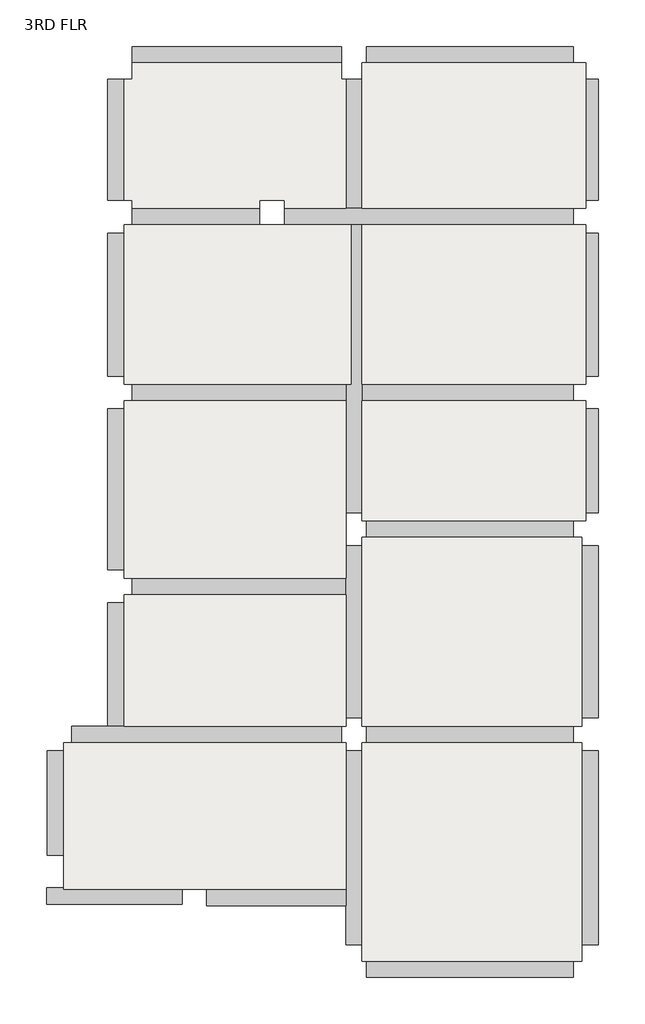
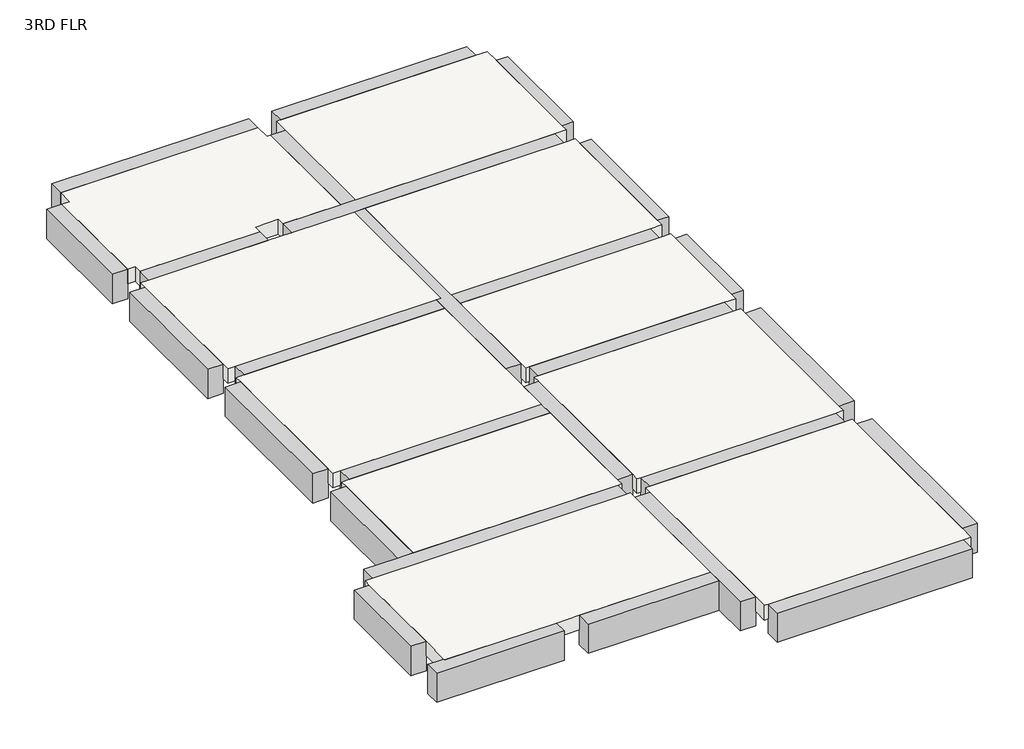
# One storey: 27 beams, 10 slabs.
"""IFC4 building model written with IfcOpenShell, lengths in millimetres."""

from ifc_helpers import new_model, si_unit, frame, origin, place, context, project, spatial, polyline, outline, extrude, faceted_brep, element, save

model = new_model("IFC4")

# Units and contexts
model_context = context("Model", 3, world=origin())
ifc_project = project(units=[si_unit("LENGTHUNIT", "METRE", prefix="MILLI")], contexts=[model_context])

# Site, building, storey
site = spatial("IfcSite", under=ifc_project)
building = spatial("IfcBuilding", under=site)
storey = spatial("IfcBuildingStorey", under=building, Name="3RD FLR", Elevation=9096.0)

# Beams
placement = place(None, origin())
element("IfcBeam", 1, ObjectType="M_Concrete-Rectangular Beam : 300 x 600mm", at=placement, inside=storey, context=model_context, shape_type="Brep", body=[
    faceted_brep([(-2096.635935, 10150.0657956, 9096.0), (-2096.635935, 10450.0657956, 9096.0), (-5925.9642664, 10450.0657956, 9096.0), (-5925.9642664, 10150.0657956, 9096.0), (-2096.635935, 10150.0657956, 8496.0), (-2096.635935, 10150.0657956, 8796.0), (-5925.9642664, 10150.0657956, 8796.0), (-5925.9642664, 10150.0657956, 8496.0), (-2096.635935, 10450.0657956, 8496.0), (-5925.9642664, 10450.0657956, 8496.0)], [[[0, 1, 2, 3]], [[4, 5, 0, 3, 6, 7]], [[8, 4, 7, 9]], [[1, 8, 9, 2]], [[2, 9, 7, 6, 3]], [[1, 0, 5, 4, 8]]]),
])
element("IfcBeam", 2, ObjectType="M_Concrete-Rectangular Beam : 300 x 600mm", at=placement, inside=storey, context=model_context, shape_type="SweptSolid", body=[
    extrude(outline(polyline([(2143.5134108, 10450.0657956), (2143.5134108, 10150.0657956), (-1646.635935, 10150.0657956), (-1646.635935, 10450.0657956), (2143.5134108, 10450.0657956)])), frame((0.0, 0.0, 8496.0), z_axis=(0.0, 0.0, 1.0), x_axis=(1.0, 0.0, 0.0)), (0.0, 0.0, 1.0), 600.0),
])
element("IfcBeam", 3, ObjectType="M_Concrete-Rectangular Beam : 300 x 600mm", at=placement, inside=storey, context=model_context, shape_type="Brep", body=[
    faceted_brep([(-6375.9642664, 7641.506653, 9096.0), (-6075.9642664, 7641.506653, 9096.0), (-6075.9642664, 9850.0657956, 9096.0), (-6375.9642664, 9850.0657956, 9096.0), (-6375.9642664, 7641.506653, 8496.0), (-6375.9642664, 9850.0657956, 8496.0), (-6075.9642664, 7641.506653, 8496.0), (-6075.9642664, 9850.0657956, 8496.0), (-6075.9642664, 7641.506653, 8796.0), (-6075.9642664, 9850.0657956, 8796.0)], [[[0, 1, 2, 3]], [[4, 0, 3, 5]], [[6, 4, 5, 7]], [[1, 8, 6, 7, 9, 2]], [[2, 9, 7, 5, 3]], [[1, 0, 4, 6, 8]]]),
])
element("IfcBeam", 4, ObjectType="M_Concrete-Rectangular Beam : 300 x 600mm", at=placement, inside=storey, context=model_context, shape_type="SweptSolid", body=[
    extrude(outline(polyline([(-6075.9642664, 4424.5351605), (-6375.9642664, 4424.5351605), (-6375.9642664, 7041.506653), (-6075.9642664, 7041.506653), (-6075.9642664, 4424.5351605)])), frame((0.0, 0.0, 8496.0), z_axis=(0.0, 0.0, 1.0), x_axis=(1.0, 0.0, 0.0)), (0.0, 0.0, 1.0), 600.0),
])
element("IfcBeam", 5, ObjectType="M_Concrete-Rectangular Beam : 300 x 600mm", at=placement, inside=storey, context=model_context, shape_type="SweptSolid", body=[
    extrude(outline(polyline([(-6075.9642664, 881.5941646), (-6375.9642664, 881.5941646), (-6375.9642664, 3824.5351605), (-6075.9642664, 3824.5351605), (-6075.9642664, 881.5941646)])), frame((0.0, 0.0, 8496.0), z_axis=(0.0, 0.0, 1.0), x_axis=(1.0, 0.0, 0.0)), (0.0, 0.0, 1.0), 600.0),
])
element("IfcBeam", 6, ObjectType="M_Concrete-Rectangular Beam : 300 x 600mm", at=placement, inside=storey, context=model_context, shape_type="SweptSolid", body=[
    extrude(outline(polyline([(2143.5134108, -6267.3380763), (2143.5134108, -6567.3380763), (-1646.635935, -6567.3380763), (-1646.635935, -6267.3380763), (2143.5134108, -6267.3380763)])), frame((0.0, 0.0, 8496.0), z_axis=(0.0, 0.0, 1.0), x_axis=(1.0, 0.0, 0.0)), (0.0, 0.0, 1.0), 600.0),
])
element("IfcBeam", 7, ObjectType="M_Concrete-Rectangular Beam : 300 x 600mm", at=placement, inside=storey, context=model_context, shape_type="SweptSolid", body=[
    extrude(outline(polyline([(2293.5134108, -2423.3693625), (2593.5134108, -2423.3693625), (2593.5134108, -5967.3380763), (2293.5134108, -5967.3380763), (2293.5134108, -2423.3693625)])), frame((0.0, 0.0, 8496.0), z_axis=(0.0, 0.0, 1.0), x_axis=(1.0, 0.0, 0.0)), (0.0, 0.0, 1.0), 600.0),
])
element("IfcBeam", 8, ObjectType="M_Concrete-Rectangular Beam : 300 x 600mm", at=placement, inside=storey, context=model_context, shape_type="SweptSolid", body=[
    extrude(outline(polyline([(2293.5134108, 1328.1057379), (2593.5134108, 1328.1057379), (2593.5134108, -1823.3693625), (2293.5134108, -1823.3693625), (2293.5134108, 1328.1057379)])), frame((0.0, 0.0, 8496.0), z_axis=(0.0, 0.0, 1.0), x_axis=(1.0, 0.0, 0.0)), (0.0, 0.0, 1.0), 600.0),
])
element("IfcBeam", 9, ObjectType="M_Concrete-Rectangular Beam : 300 x 600mm", at=placement, inside=storey, context=model_context, shape_type="SweptSolid", body=[
    extrude(outline(polyline([(8496.0, 2293.5134108), (8496.0, 2593.5134108), (9096.0, 2593.5134108), (9096.0, 2368.5134108), (8796.0, 2368.5134108), (8796.0, 2293.5134108), (8496.0, 2293.5134108)])), frame((0.0, 1928.1057379, 0.0), z_axis=(0.0, 1.0, 0.0), x_axis=(0.0, 0.0, 1.0)), (0.0, 0.0, 1.0), 1896.4294226),
])
element("IfcBeam", 10, ObjectType="M_Concrete-Rectangular Beam : 300 x 600mm", at=placement, inside=storey, context=model_context, shape_type="SweptSolid", body=[
    extrude(outline(polyline([(8496.0, 2293.5134108), (8496.0, 2593.5134108), (9096.0, 2593.5134108), (9096.0, 2368.5134108), (8796.0, 2368.5134108), (8796.0, 2293.5134108), (8496.0, 2293.5134108)])), frame((0.0, 4424.5351605, 0.0), z_axis=(0.0, 1.0, 0.0), x_axis=(0.0, 0.0, 1.0)), (0.0, 0.0, 1.0), 2616.9714925),
])
element("IfcBeam", 11, ObjectType="M_Concrete-Rectangular Beam : 300 x 600mm", at=placement, inside=storey, context=model_context, shape_type="SweptSolid", body=[
    extrude(outline(polyline([(8496.0, 2293.5134108), (8496.0, 2593.5134108), (9096.0, 2593.5134108), (9096.0, 2368.5134108), (8796.0, 2368.5134108), (8796.0, 2293.5134108), (8496.0, 2293.5134108)])), frame((0.0, 7641.506653, 0.0), z_axis=(0.0, 1.0, 0.0), x_axis=(0.0, 0.0, 1.0)), (0.0, 0.0, 1.0), 2208.5591426),
])
element("IfcBeam", 12, ObjectType="M_Concrete-Rectangular Beam : 300 x 600mm", at=placement, inside=storey, context=model_context, shape_type="Brep", body=[
    faceted_brep([(-3596.635935, 7191.506653, 9096.0), (-3596.635935, 7491.506653, 9096.0), (-5925.9642664, 7491.506653, 9096.0), (-5925.9642664, 7191.506653, 9096.0), (-3596.635935, 7191.506653, 8496.0), (-5925.9642664, 7191.506653, 8496.0), (-3596.635935, 7491.506653, 8496.0), (-5925.9642664, 7491.506653, 8496.0), (-3596.635935, 7491.506653, 8796.0), (-5925.9642664, 7491.506653, 8796.0)], [[[0, 1, 2, 3]], [[4, 0, 3, 5]], [[6, 4, 5, 7]], [[1, 8, 6, 7, 9, 2]], [[2, 9, 7, 5, 3]], [[1, 0, 4, 6, 8]]]),
])
element("IfcBeam", 13, ObjectType="M_Concrete-Rectangular Beam : 300 x 600mm", at=placement, inside=storey, context=model_context, shape_type="Brep", body=[
    faceted_brep([(-3146.635935, 7491.506653, 9096.0), (-3146.635935, 7191.506653, 9096.0), (-1928.7254278, 7191.506653, 9096.0), (-1721.635935, 7191.506653, 9096.0), (2143.5134108, 7191.506653, 9096.0), (2143.5134108, 7491.506653, 9096.0), (-1721.635935, 7491.506653, 9096.0), (-2021.635935, 7491.506653, 9096.0), (-3146.635935, 7491.506653, 8496.0), (-3146.635935, 7491.506653, 8796.0), (2143.5134108, 7491.506653, 8496.0), (-1721.635935, 7491.506653, 8496.0), (-2021.635935, 7491.506653, 8496.0), (-3146.635935, 7191.506653, 8496.0), (2143.5134108, 7191.506653, 8496.0), (-1721.635935, 7191.506653, 8496.0), (-2021.635935, 7191.506653, 8496.0)], [[[0, 1, 2, 3, 4, 5, 6, 7]], [[8, 9, 0, 7, 6, 5, 10, 11, 12]], [[13, 8, 12, 11, 10, 14, 15, 16]], [[1, 13, 16, 15, 14, 4, 3, 2]], [[1, 0, 9, 8, 13]], [[4, 14, 10, 5]]]),
])
element("IfcBeam", 14, ObjectType="M_Concrete-Rectangular Beam : 300 x 600mm", at=placement, inside=storey, context=model_context, shape_type="SweptSolid", body=[
    extrude(outline(polyline([(-1646.635935, 1478.1057379), (-1646.635935, 1778.1057379), (2143.5134108, 1778.1057379), (2143.5134108, 1478.1057379), (-1646.635935, 1478.1057379)])), frame((0.0, 0.0, 8496.0), z_axis=(0.0, 0.0, 1.0), x_axis=(1.0, 0.0, 0.0)), (0.0, 0.0, 1.0), 600.0),
])
element("IfcBeam", 15, ObjectType="M_Concrete-Rectangular Beam : 300 x 600mm", at=placement, inside=storey, context=model_context, shape_type="SweptSolid", body=[
    extrude(outline(polyline([(-1646.635935, -2273.3693625), (-1646.635935, -1973.3693625), (2143.5134108, -1973.3693625), (2143.5134108, -2273.3693625), (-1646.635935, -2273.3693625)])), frame((0.0, 0.0, 8496.0), z_axis=(0.0, 0.0, 1.0), x_axis=(1.0, 0.0, 0.0)), (0.0, 0.0, 1.0), 600.0),
])
element("IfcBeam", 16, ObjectType="M_Concrete-Rectangular Beam : 300 x 600mm", at=placement, inside=storey, context=model_context, shape_type="Brep", body=[
    faceted_brep([(-1721.635935, -2423.3693625, 9096.0), (-2021.635935, -2423.3693625, 9096.0), (-2021.635935, -4959.2575036, 9096.0), (-2021.635935, -5259.2575036, 9096.0), (-2021.635935, -5967.3380763, 9096.0), (-1721.635935, -5967.3380763, 9096.0), (-1721.635935, -2423.3693625, 8496.0), (-1721.635935, -5967.3380763, 8496.0), (-2021.635935, -2423.3693625, 8496.0), (-2021.635935, -5967.3380763, 8496.0), (-2021.635935, -5259.2575036, 8496.0), (-2021.635935, -4959.2575036, 8496.0)], [[[0, 1, 2, 3, 4, 5]], [[6, 0, 5, 7]], [[8, 6, 7, 9, 10, 11]], [[1, 8, 11, 10, 9, 4, 3, 2]], [[1, 0, 6, 8]], [[4, 9, 7, 5]]]),
])
element("IfcBeam", 17, ObjectType="M_Concrete-Rectangular Beam : 300 x 600mm", at=placement, inside=storey, context=model_context, shape_type="Brep", body=[
    faceted_brep([(-1721.635935, 1328.1057379, 9096.0), (-2021.635935, 1328.1057379, 9096.0), (-2021.635935, 731.5941646, 9096.0), (-2021.635935, 431.5941646, 9096.0), (-2021.635935, -1823.3693625, 9096.0), (-1721.635935, -1823.3693625, 9096.0), (-1721.635935, 1328.1057379, 8496.0), (-1721.635935, -1823.3693625, 8496.0), (-2021.635935, 1328.1057379, 8496.0), (-2021.635935, -1823.3693625, 8496.0), (-2021.635935, 431.5941646, 8496.0), (-2021.635935, 731.5941646, 8496.0)], [[[0, 1, 2, 3, 4, 5]], [[6, 0, 5, 7]], [[8, 6, 7, 9, 10, 11]], [[1, 8, 11, 10, 9, 4, 3, 2]], [[1, 0, 6, 8]], [[4, 9, 7, 5]]]),
])
element("IfcBeam", 18, ObjectType="M_Concrete-Rectangular Beam : 300 x 600mm", at=placement, inside=storey, context=model_context, shape_type="Brep", body=[
    faceted_brep([(-4566.635935, -4959.2575036, 9096.0), (-4566.635935, -5259.2575036, 9096.0), (-2021.635935, -5259.2575036, 9096.0), (-2021.635935, -4959.2575036, 9096.0), (-4566.635935, -5259.2575036, 8496.0), (-2021.635935, -5259.2575036, 8496.0), (-4566.635935, -4959.2575036, 8496.0), (-2021.635935, -4959.2575036, 8496.0), (-2021.635935, -4959.2575036, 8796.0)], [[[0, 1, 2, 3]], [[1, 4, 5, 2]], [[4, 6, 7, 5]], [[6, 0, 3, 8, 7]], [[0, 6, 4, 1]], [[3, 2, 5, 7, 8]]]),
])
element("IfcBeam", 19, ObjectType="M_Concrete-Rectangular Beam : 300 x 600mm", at=placement, inside=storey, context=model_context, shape_type="Brep", body=[
    faceted_brep([(-7032.9642664, -1973.3693625, 9096.0), (-7032.9642664, -2273.3693625, 9096.0), (-2096.635935, -2273.3693625, 9096.0), (-2096.635935, -1973.3693625, 9096.0), (-6075.9642664, -1973.3693625, 9096.0), (-6375.9642664, -1973.3693625, 9096.0), (-7032.9642664, -1973.3693625, 8496.0), (-2096.635935, -1973.3693625, 8496.0), (-6075.9642664, -1973.3693625, 8496.0), (-6375.9642664, -1973.3693625, 8496.0), (-7032.9642664, -2273.3693625, 8496.0), (-2096.635935, -2273.3693625, 8496.0)], [[[0, 1, 2, 3, 4, 5]], [[6, 0, 5, 4, 3, 7, 8, 9]], [[10, 6, 9, 8, 7, 11]], [[1, 10, 11, 2]], [[2, 11, 7, 3]], [[1, 0, 6, 10]]]),
])
element("IfcBeam", 20, ObjectType="M_Concrete-Rectangular Beam : 300 x 600mm", at=placement, inside=storey, context=model_context, shape_type="Brep", body=[
    faceted_brep([(-6075.9642664, 281.5941646, 9096.0), (-6375.9642664, 281.5941646, 9096.0), (-6375.9642664, -1973.3693625, 9096.0), (-6075.9642664, -1973.3693625, 9096.0), (-6375.9642664, 281.5941646, 8496.0), (-6375.9642664, -1973.3693625, 8496.0), (-6075.9642664, 281.5941646, 8496.0), (-6075.9642664, -1973.3693625, 8496.0), (-6075.9642664, -1973.3693625, 8796.0)], [[[0, 1, 2, 3]], [[1, 4, 5, 2]], [[4, 6, 7, 5]], [[6, 0, 3, 8, 7]], [[0, 6, 4, 1]], [[3, 2, 5, 7, 8]]]),
])
element("IfcBeam", 21, ObjectType="M_Concrete-Rectangular Beam : 300 x 600mm", at=placement, inside=storey, context=model_context, shape_type="SweptSolid", body=[
    extrude(outline(polyline([(-7182.9642664, -4329.2575036), (-7482.9642664, -4329.2575036), (-7482.9642664, -2423.3693625), (-7182.9642664, -2423.3693625), (-7182.9642664, -4329.2575036)])), frame((0.0, 0.0, 8496.0), z_axis=(0.0, 0.0, 1.0), x_axis=(1.0, 0.0, 0.0)), (0.0, 0.0, 1.0), 600.0),
])
element("IfcBeam", 22, ObjectType="M_Concrete-Rectangular Beam : 300 x 600mm", at=placement, inside=storey, context=model_context, shape_type="Brep", body=[
    faceted_brep([(-7496.635935, -5229.2575036, 9096.0), (-7496.635935, -4929.2575036, 9096.0), (-7496.635935, -4929.2575036, 8496.0), (-7496.635935, -5229.2575036, 8496.0), (-5016.635935, -5229.2575036, 9096.0), (-5016.635935, -4959.2575036, 9096.0), (-7182.9642664, -4959.2575036, 9096.0), (-7182.9642664, -4929.2575036, 9096.0), (-7482.9642664, -4929.2575036, 9096.0), (-7182.9642664, -4929.2575036, 8796.0), (-7032.9642664, -4929.2575036, 8796.0), (-5016.635935, -4929.2575036, 8796.0), (-5016.635935, -4929.2575036, 8496.0), (-5016.635935, -5229.2575036, 8496.0), (-5016.635935, -4959.2575036, 8796.0), (-7182.9642664, -4959.2575036, 8796.0)], [[[0, 1, 2, 3]], [[1, 0, 4, 5, 6, 7, 8]], [[2, 1, 8, 7, 9, 10, 11, 12]], [[3, 2, 12, 13]], [[0, 3, 13, 4]], [[4, 13, 12, 11, 14, 5]], [[9, 15, 14, 11, 10]], [[15, 6, 5, 14]], [[6, 15, 9, 7]]]),
])
element("IfcBeam", 23, ObjectType="M_Concrete-Rectangular Beam : 300 x 600mm", at=placement, inside=storey, context=model_context, shape_type="Brep", body=[
    faceted_brep([(-1721.635935, 9850.0657956, 9096.0), (-2021.635935, 9850.0657956, 9096.0), (-2021.635935, 7491.506653, 9096.0), (-1721.635935, 7491.506653, 9096.0), (-2021.635935, 9850.0657956, 8796.0), (-2021.635935, 9850.0657956, 8496.0), (-2021.635935, 7491.506653, 8496.0), (-2021.635935, 7491.506653, 8796.0), (-1721.635935, 9850.0657956, 8496.0), (-1721.635935, 7491.506653, 8496.0), (-1721.635935, 7491.506653, 8796.0)], [[[0, 1, 2, 3]], [[1, 4, 5, 6, 7, 2]], [[5, 8, 9, 6]], [[8, 0, 3, 10, 9]], [[0, 8, 5, 4, 1]], [[3, 2, 7, 6, 9, 10]]]),
])
element("IfcBeam", 24, ObjectType="M_Concrete-Rectangular Beam : 300 x 600mm", at=placement, inside=storey, context=model_context, shape_type="Brep", body=[
    faceted_brep([(-2021.635935, 1928.1057379, 9096.0), (-1721.635935, 1928.1057379, 9096.0), (-1721.635935, 3974.5351605, 9096.0), (-1721.635935, 4274.5351605, 9096.0), (-1721.635935, 7191.506653, 9096.0), (-1928.7254278, 7191.506653, 9096.0), (-1928.7254278, 4274.5351605, 9096.0), (-2021.635935, 4274.5351605, 9096.0), (-2021.635935, 3974.5351605, 9096.0), (-1721.635935, 1928.1057379, 8496.0), (-1721.635935, 3974.5351605, 8496.0), (-1721.635935, 4274.5351605, 8496.0), (-1721.635935, 7191.506653, 8496.0), (-1721.635935, 7191.506653, 8796.0), (-2021.635935, 1928.1057379, 8496.0), (-2021.635935, 3974.5351605, 8496.0), (-2021.635935, 4274.5351605, 8496.0), (-2021.635935, 7191.506653, 8496.0), (-2021.635935, 4274.5351605, 8796.0), (-2021.635935, 7191.506653, 8796.0), (-1928.7254278, 7191.506653, 8796.0), (-1928.7254278, 4274.5351605, 8796.0)], [[[0, 1, 2, 3, 4, 5, 6, 7, 8]], [[1, 9, 10, 11, 12, 13, 4, 3, 2]], [[9, 14, 15, 16, 17, 12, 11, 10]], [[14, 0, 8, 7, 18, 19, 17, 16, 15]], [[0, 14, 9, 1]], [[4, 13, 12, 17, 19, 20, 5]], [[21, 20, 19, 18]], [[20, 21, 6, 5]], [[6, 21, 18, 7]]]),
])
element("IfcBeam", 25, ObjectType="M_Concrete-Rectangular Beam : 300 x 600mm", at=placement, inside=storey, context=model_context, shape_type="Brep", body=[
    faceted_brep([(-5925.9642664, 731.5941646, 9096.0), (-5925.9642664, 431.5941646, 9096.0), (-2021.635935, 431.5941646, 9096.0), (-2021.635935, 731.5941646, 9096.0), (-5925.9642664, 431.5941646, 8496.0), (-2021.635935, 431.5941646, 8496.0), (-2021.635935, 431.5941646, 8796.0), (-5925.9642664, 731.5941646, 8496.0), (-2021.635935, 731.5941646, 8496.0), (-2021.635935, 731.5941646, 8796.0)], [[[0, 1, 2, 3]], [[1, 4, 5, 6, 2]], [[4, 7, 8, 5]], [[7, 0, 3, 9, 8]], [[0, 7, 4, 1]], [[3, 2, 6, 5, 8, 9]]]),
])
element("IfcBeam", 26, ObjectType="M_Concrete-Rectangular Beam : 300 x 600mm", at=placement, inside=storey, context=model_context, shape_type="Brep", body=[
    faceted_brep([(-5925.9642664, 4274.5351605, 9096.0), (-5925.9642664, 3974.5351605, 9096.0), (-2021.635935, 3974.5351605, 9096.0), (-2021.635935, 4274.5351605, 9096.0), (-5925.9642664, 3974.5351605, 8496.0), (-2021.635935, 3974.5351605, 8496.0), (-2021.635935, 3974.5351605, 8796.0), (-5925.9642664, 4274.5351605, 8496.0), (-2021.635935, 4274.5351605, 8496.0), (-2021.635935, 4274.5351605, 8796.0)], [[[0, 1, 2, 3]], [[1, 4, 5, 6, 2]], [[4, 7, 8, 5]], [[7, 0, 3, 9, 8]], [[0, 7, 4, 1]], [[3, 2, 6, 5, 8, 9]]]),
])
element("IfcBeam", 27, ObjectType="M_Concrete-Rectangular Beam : 300 x 600mm", at=placement, inside=storey, context=model_context, shape_type="Brep", body=[
    faceted_brep([(2143.5134108, 3974.5351605, 9096.0), (2143.5134108, 4274.5351605, 9096.0), (-1721.635935, 4274.5351605, 9096.0), (-1721.635935, 3974.5351605, 9096.0), (2143.5134108, 4274.5351605, 8496.0), (-1721.635935, 4274.5351605, 8496.0), (-1721.635935, 4274.5351605, 8796.0), (2143.5134108, 3974.5351605, 8496.0), (-1721.635935, 3974.5351605, 8496.0), (-1721.635935, 3974.5351605, 8796.0)], [[[0, 1, 2, 3]], [[1, 4, 5, 6, 2]], [[4, 7, 8, 5]], [[7, 0, 3, 9, 8]], [[0, 7, 4, 1]], [[3, 2, 6, 5, 8, 9]]]),
])

# Slabs
element("IfcSlab", 28, ObjectType="Generic 300mm", at=placement, inside=storey, context=model_context, shape_type="SweptSolid", body=[
    extrude(outline(polyline([(-2096.635935, 10150.0657956), (-2096.635935, 9850.0657956), (-2021.635935, 9850.0657956), (-2021.635935, 7491.506653), (-3146.635935, 7491.506653), (-3146.635935, 7641.506653), (-3596.635935, 7641.506653), (-3596.635935, 7491.506653), (-5925.9642664, 7491.506653), (-5925.9642664, 7641.506653), (-6075.9642664, 7641.506653), (-6075.9642664, 9850.0657956), (-5925.9642664, 9850.0657956), (-5925.9642664, 10150.0657956), (-2096.635935, 10150.0657956)])), frame((0.0, 0.0, 8796.0), z_axis=(0.0, 0.0, 1.0), x_axis=(1.0, 0.0, 0.0)), (0.0, 0.0, 1.0), 300.0),
])
element("IfcSlab", 29, ObjectType="Generic 300mm", at=placement, inside=storey, context=model_context, shape_type="Brep", body=[
    faceted_brep([(-1721.635935, 10150.0657956, 8796.0), (-1646.635935, 10150.0657956, 8796.0), (2143.5134108, 10150.0657956, 8796.0), (2368.5134108, 10150.0657956, 8796.0), (2368.5134108, 9850.0657956, 8796.0), (2368.5134108, 7641.506653, 8796.0), (2368.5134108, 7491.506653, 8796.0), (2143.5134108, 7491.506653, 8796.0), (-1721.635935, 7491.506653, 8796.0), (-1721.635935, 9850.0657956, 8796.0), (-1721.635935, 10150.0657956, 9096.0), (-1721.635935, 9850.0657956, 9096.0), (-1721.635935, 7491.506653, 9096.0), (2143.5134108, 7491.506653, 9096.0), (2368.5134108, 7491.506653, 9096.0), (2368.5134108, 7641.506653, 9096.0), (2368.5134108, 9850.0657956, 9096.0), (2368.5134108, 10150.0657956, 9096.0), (2143.5134108, 10150.0657956, 9096.0), (-1646.635935, 10150.0657956, 9096.0)], [[[0, 1, 2, 3, 4, 5, 6, 7, 8, 9]], [[10, 11, 12, 13, 14, 15, 16, 17, 18, 19]], [[3, 2, 1, 0, 10, 19, 18, 17]], [[6, 5, 4, 3, 17, 16, 15, 14]], [[8, 7, 6, 14, 13, 12]], [[0, 9, 8, 12, 11, 10]]]),
])
element("IfcSlab", 30, ObjectType="Generic 300mm", at=placement, inside=storey, context=model_context, shape_type="Brep", body=[
    faceted_brep([(-1721.635935, 7191.506653, 8796.0), (2143.5134108, 7191.506653, 8796.0), (2368.5134108, 7191.506653, 8796.0), (2368.5134108, 7041.506653, 8796.0), (2368.5134108, 4424.5351605, 8796.0), (2368.5134108, 4274.5351605, 8796.0), (2143.5134108, 4274.5351605, 8796.0), (-1721.635935, 4274.5351605, 8796.0), (-1721.635935, 7191.506653, 9096.0), (-1721.635935, 4274.5351605, 9096.0), (2143.5134108, 4274.5351605, 9096.0), (2368.5134108, 4274.5351605, 9096.0), (2368.5134108, 4424.5351605, 9096.0), (2368.5134108, 7041.506653, 9096.0), (2368.5134108, 7191.506653, 9096.0), (2143.5134108, 7191.506653, 9096.0)], [[[0, 1, 2, 3, 4, 5, 6, 7]], [[8, 9, 10, 11, 12, 13, 14, 15]], [[2, 1, 0, 8, 15, 14]], [[5, 4, 3, 2, 14, 13, 12, 11]], [[7, 6, 5, 11, 10, 9]], [[0, 7, 9, 8]]]),
])
element("IfcSlab", 31, ObjectType="Generic 300mm", at=placement, inside=storey, context=model_context, shape_type="Brep", body=[
    faceted_brep([(-6075.9642664, 7191.506653, 8796.0), (-5925.9642664, 7191.506653, 8796.0), (-3596.635935, 7191.506653, 8796.0), (-3146.635935, 7191.506653, 8796.0), (-2021.635935, 7191.506653, 8796.0), (-1928.7254278, 7191.506653, 8796.0), (-1928.7254278, 4274.5351605, 8796.0), (-2021.635935, 4274.5351605, 8796.0), (-5925.9642664, 4274.5351605, 8796.0), (-6075.9642664, 4274.5351605, 8796.0), (-6075.9642664, 4424.5351605, 8796.0), (-6075.9642664, 7041.506653, 8796.0), (-6075.9642664, 7191.506653, 9096.0), (-6075.9642664, 7041.506653, 9096.0), (-6075.9642664, 4424.5351605, 9096.0), (-6075.9642664, 4274.5351605, 9096.0), (-5925.9642664, 4274.5351605, 9096.0), (-2021.635935, 4274.5351605, 9096.0), (-1928.7254278, 4274.5351605, 9096.0), (-1928.7254278, 7191.506653, 9096.0), (-3146.635935, 7191.506653, 9096.0), (-3596.635935, 7191.506653, 9096.0), (-5925.9642664, 7191.506653, 9096.0)], [[[0, 1, 2, 3, 4, 5, 6, 7, 8, 9, 10, 11]], [[12, 13, 14, 15, 16, 17, 18, 19, 20, 21, 22]], [[5, 4, 3, 2, 1, 0, 12, 22, 21, 20, 19]], [[6, 5, 19, 18]], [[9, 8, 7, 6, 18, 17, 16, 15]], [[0, 11, 10, 9, 15, 14, 13, 12]]]),
])
element("IfcSlab", 32, ObjectType="Generic 300mm", at=placement, inside=storey, context=model_context, shape_type="Brep", body=[
    faceted_brep([(-1721.635935, 3974.5351605, 8796.0), (2143.5134108, 3974.5351605, 8796.0), (2368.5134108, 3974.5351605, 8796.0), (2368.5134108, 3824.5351605, 8796.0), (2368.5134108, 1928.1057379, 8796.0), (2368.5134108, 1778.1057379, 8796.0), (2143.5134108, 1778.1057379, 8796.0), (-1646.635935, 1778.1057379, 8796.0), (-1721.635935, 1778.1057379, 8796.0), (-1721.635935, 1928.1057379, 8796.0), (-1721.635935, 3974.5351605, 9096.0), (-1721.635935, 1928.1057379, 9096.0), (-1721.635935, 1778.1057379, 9096.0), (-1646.635935, 1778.1057379, 9096.0), (2143.5134108, 1778.1057379, 9096.0), (2368.5134108, 1778.1057379, 9096.0), (2368.5134108, 1928.1057379, 9096.0), (2368.5134108, 3824.5351605, 9096.0), (2368.5134108, 3974.5351605, 9096.0), (2143.5134108, 3974.5351605, 9096.0)], [[[0, 1, 2, 3, 4, 5, 6, 7, 8, 9]], [[10, 11, 12, 13, 14, 15, 16, 17, 18, 19]], [[2, 1, 0, 10, 19, 18]], [[5, 4, 3, 2, 18, 17, 16, 15]], [[8, 7, 6, 5, 15, 14, 13, 12]], [[0, 9, 8, 12, 11, 10]]]),
])
element("IfcSlab", 33, ObjectType="Generic 300mm", at=placement, inside=storey, context=model_context, shape_type="Brep", body=[
    faceted_brep([(-1721.635935, 1478.1057379, 8796.0), (-1646.635935, 1478.1057379, 8796.0), (2143.5134108, 1478.1057379, 8796.0), (2293.5134108, 1478.1057379, 8796.0), (2293.5134108, 1328.1057379, 8796.0), (2293.5134108, -1823.3693625, 8796.0), (2293.5134108, -1973.3693625, 8796.0), (2143.5134108, -1973.3693625, 8796.0), (-1646.635935, -1973.3693625, 8796.0), (-1721.635935, -1973.3693625, 8796.0), (-1721.635935, -1823.3693625, 8796.0), (-1721.635935, 1328.1057379, 8796.0), (-1721.635935, 1478.1057379, 9096.0), (-1721.635935, 1328.1057379, 9096.0), (-1721.635935, -1823.3693625, 9096.0), (-1721.635935, -1973.3693625, 9096.0), (-1646.635935, -1973.3693625, 9096.0), (2143.5134108, -1973.3693625, 9096.0), (2293.5134108, -1973.3693625, 9096.0), (2293.5134108, -1823.3693625, 9096.0), (2293.5134108, 1328.1057379, 9096.0), (2293.5134108, 1478.1057379, 9096.0), (2143.5134108, 1478.1057379, 9096.0), (-1646.635935, 1478.1057379, 9096.0)], [[[0, 1, 2, 3, 4, 5, 6, 7, 8, 9, 10, 11]], [[12, 13, 14, 15, 16, 17, 18, 19, 20, 21, 22, 23]], [[3, 2, 1, 0, 12, 23, 22, 21]], [[6, 5, 4, 3, 21, 20, 19, 18]], [[9, 8, 7, 6, 18, 17, 16, 15]], [[0, 11, 10, 9, 15, 14, 13, 12]]]),
])
element("IfcSlab", 34, ObjectType="Generic 300mm", at=placement, inside=storey, context=model_context, shape_type="Brep", body=[
    faceted_brep([(-1721.635935, -2273.3693625, 8796.0), (-1646.635935, -2273.3693625, 8796.0), (2143.5134108, -2273.3693625, 8796.0), (2293.5134108, -2273.3693625, 8796.0), (2293.5134108, -2423.3693625, 8796.0), (2293.5134108, -5967.3380763, 8796.0), (2293.5134108, -6267.3380763, 8796.0), (2143.5134108, -6267.3380763, 8796.0), (-1646.635935, -6267.3380763, 8796.0), (-1721.635935, -6267.3380763, 8796.0), (-1721.635935, -5967.3380763, 8796.0), (-1721.635935, -2423.3693625, 8796.0), (-1721.635935, -2273.3693625, 9096.0), (-1721.635935, -2423.3693625, 9096.0), (-1721.635935, -5967.3380763, 9096.0), (-1721.635935, -6267.3380763, 9096.0), (-1646.635935, -6267.3380763, 9096.0), (2143.5134108, -6267.3380763, 9096.0), (2293.5134108, -6267.3380763, 9096.0), (2293.5134108, -5967.3380763, 9096.0), (2293.5134108, -2423.3693625, 9096.0), (2293.5134108, -2273.3693625, 9096.0), (2143.5134108, -2273.3693625, 9096.0), (-1646.635935, -2273.3693625, 9096.0)], [[[0, 1, 2, 3, 4, 5, 6, 7, 8, 9, 10, 11]], [[12, 13, 14, 15, 16, 17, 18, 19, 20, 21, 22, 23]], [[3, 2, 1, 0, 12, 23, 22, 21]], [[6, 5, 4, 3, 21, 20, 19, 18]], [[9, 8, 7, 6, 18, 17, 16, 15]], [[0, 11, 10, 9, 15, 14, 13, 12]]]),
])
element("IfcSlab", 35, ObjectType="Generic 300mm", at=placement, inside=storey, context=model_context, shape_type="Brep", body=[
    faceted_brep([(-6075.9642664, 3974.5351605, 8796.0), (-5925.9642664, 3974.5351605, 8796.0), (-2021.635935, 3974.5351605, 8796.0), (-2021.635935, 1928.1057379, 8796.0), (-2021.635935, 1328.1057379, 8796.0), (-2021.635935, 731.5941646, 8796.0), (-5925.9642664, 731.5941646, 8796.0), (-6075.9642664, 731.5941646, 8796.0), (-6075.9642664, 881.5941646, 8796.0), (-6075.9642664, 3824.5351605, 8796.0), (-6075.9642664, 3974.5351605, 9096.0), (-6075.9642664, 3824.5351605, 9096.0), (-6075.9642664, 881.5941646, 9096.0), (-6075.9642664, 731.5941646, 9096.0), (-5925.9642664, 731.5941646, 9096.0), (-2021.635935, 731.5941646, 9096.0), (-2021.635935, 1328.1057379, 9096.0), (-2021.635935, 1928.1057379, 9096.0), (-2021.635935, 3974.5351605, 9096.0), (-5925.9642664, 3974.5351605, 9096.0)], [[[0, 1, 2, 3, 4, 5, 6, 7, 8, 9]], [[10, 11, 12, 13, 14, 15, 16, 17, 18, 19]], [[2, 1, 0, 10, 19, 18]], [[5, 4, 3, 2, 18, 17, 16, 15]], [[7, 6, 5, 15, 14, 13]], [[0, 9, 8, 7, 13, 12, 11, 10]]]),
])
element("IfcSlab", 36, ObjectType="Generic 300mm", at=placement, inside=storey, context=model_context, shape_type="Brep", body=[
    faceted_brep([(-6075.9642664, 431.5941646, 8796.0), (-5925.9642664, 431.5941646, 8796.0), (-2021.635935, 431.5941646, 8796.0), (-2021.635935, -1823.3693625, 8796.0), (-2021.635935, -1973.3693625, 8796.0), (-2096.635935, -1973.3693625, 8796.0), (-6075.9642664, -1973.3693625, 8796.0), (-6075.9642664, 281.5941646, 8796.0), (-6075.9642664, 431.5941646, 9096.0), (-6075.9642664, 281.5941646, 9096.0), (-6075.9642664, -1973.3693625, 9096.0), (-2096.635935, -1973.3693625, 9096.0), (-2021.635935, -1973.3693625, 9096.0), (-2021.635935, -1823.3693625, 9096.0), (-2021.635935, 431.5941646, 9096.0), (-5925.9642664, 431.5941646, 9096.0)], [[[0, 1, 2, 3, 4, 5, 6, 7]], [[8, 9, 10, 11, 12, 13, 14, 15]], [[2, 1, 0, 8, 15, 14]], [[4, 3, 2, 14, 13, 12]], [[6, 5, 4, 12, 11, 10]], [[0, 7, 6, 10, 9, 8]]]),
])
element("IfcSlab", 37, ObjectType="Generic 300mm", at=placement, inside=storey, context=model_context, shape_type="Brep", body=[
    faceted_brep([(-7182.9642664, -2273.3693625, 8796.0), (-7032.9642664, -2273.3693625, 8796.0), (-2096.635935, -2273.3693625, 8796.0), (-2021.635935, -2273.3693625, 8796.0), (-2021.635935, -2423.3693625, 8796.0), (-2021.635935, -4959.2575036, 8796.0), (-4566.635935, -4959.2575036, 8796.0), (-5016.635935, -4959.2575036, 8796.0), (-7182.9642664, -4959.2575036, 8796.0), (-7182.9642664, -4929.2575036, 8796.0), (-7182.9642664, -4329.2575036, 8796.0), (-7182.9642664, -2423.3693625, 8796.0), (-7182.9642664, -2273.3693625, 9096.0), (-7182.9642664, -2423.3693625, 9096.0), (-7182.9642664, -4329.2575036, 9096.0), (-7182.9642664, -4929.2575036, 9096.0), (-7182.9642664, -4959.2575036, 9096.0), (-5016.635935, -4959.2575036, 9096.0), (-4566.635935, -4959.2575036, 9096.0), (-2021.635935, -4959.2575036, 9096.0), (-2021.635935, -2423.3693625, 9096.0), (-2021.635935, -2273.3693625, 9096.0), (-2096.635935, -2273.3693625, 9096.0), (-7032.9642664, -2273.3693625, 9096.0)], [[[0, 1, 2, 3, 4, 5, 6, 7, 8, 9, 10, 11]], [[12, 13, 14, 15, 16, 17, 18, 19, 20, 21, 22, 23]], [[3, 2, 1, 0, 12, 23, 22, 21]], [[5, 4, 3, 21, 20, 19]], [[8, 7, 6, 5, 19, 18, 17, 16]], [[0, 11, 10, 9, 8, 16, 15, 14, 13, 12]]]),
])

save(model, "model.ifc")

# Revit data of these elements
# Type "M_Concrete-Rectangular Beam : 300 x 600mm"
#   Length [instance default] = 1524 mm
#   b = 300 mm
#   h = 600 mm
#   Structural Material [instance default] = Concrete, Cast-in-Place gray
#   Assembly Code = ""
# Type "Generic 300mm"
#   Function = 0
#   Layers, outside or top first: 300 mm no material (function 1)
# Elements 1, 2, 3, 4, 5, 6, 7, 8, 9, 10, 11, 12, 13, 14, 15, 16, 17, 18, 19, 20, 21, 22, 23, 24, 25, 26, 27 (IfcBeam, "M_Concrete-Rectangular Beam : 300 x 600mm")
#   Structural Material = Concrete, Cast-in-Place gray
#   Phase Created = New Construction
#   Materials on its faces: "Concrete, Cast-in-Place gray"
# Element 28 (IfcSlab, "Generic 300mm")
#   Height Offset From Level = 0 mm
#   built-in parameter 1001954 = 1
#   Phase Created = New Construction
#   Materials on its faces: "Default Floor"
# Elements 29, 30, 31, 32, 33, 34, 35, 36, 37 (IfcSlab, "Generic 300mm")
#   built-in parameter 1001955 = 3.14159 (stored number, unit not read)
#   Height Offset From Level = 0 mm
#   built-in parameter 1001954 = 1
#   Phase Created = New Construction
#   Materials on its faces: "Default Floor"
# Materials
#   "Concrete, Cast-in-Place gray": class "Concrete", colour RGB 192 192 192, transparency 0, Description = "Cast-in-place concrete", Cost = 0
#   "Default Floor": colour RGB 127 127 127, transparency 0, Cost = 0
